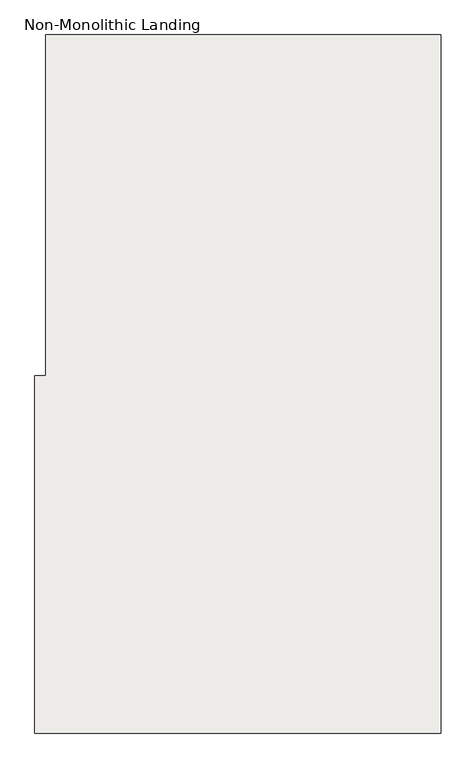
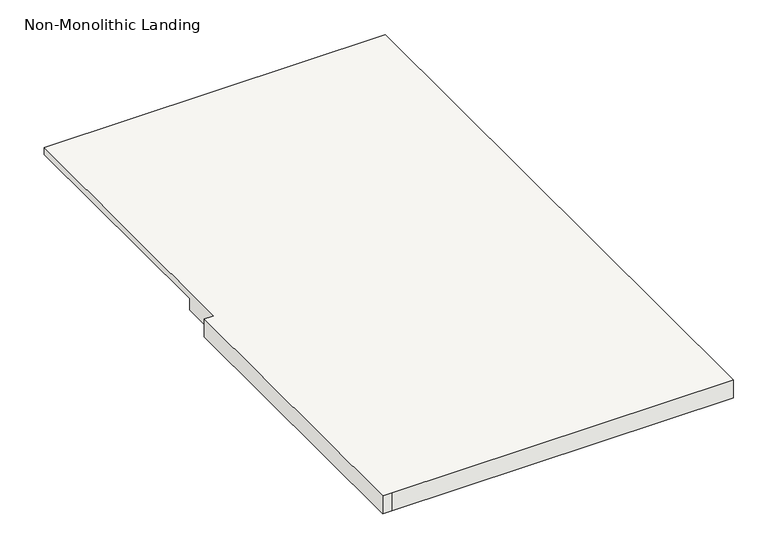
"""IFC4 building model written with IfcOpenShell, lengths in millimetres: slab geometry, Non-Monolithic Landing."""

from ifc_helpers import new_model, si_unit, origin, place, context, project, spatial, faceted_brep, source, transform, mapped, element, save


def non_monolithic_landing_dc928896(model_context):
    return source(origin(), model_context, "Body", "Brep", [
        faceted_brep([(-2950.6837185, -6386.6877785, 1581.15), (-2925.2837185, -6386.6877785, 1555.75), (-2925.2837185, -7060.9366292, 1555.75), (-2950.6837185, -7060.9366292, 1581.15), (-2950.6837185, -7174.0877785, 1600.2), (-2976.0837185, -7174.0877785, 1600.2), (-2976.0837185, -8000.7366292, 1600.2), (-2950.6837185, -8000.7366292, 1600.2), (-2036.2837185, -8000.7366292, 1600.2), (-2036.2837185, -6386.6877785, 1600.2), (-2950.6837185, -6386.6877785, 1600.2), (-2925.2837185, -7060.9366292, 1549.4), (-2925.2837185, -6386.6877785, 1549.4), (-2036.2837185, -6386.6877785, 1549.4), (-2036.2837185, -8000.7366292, 1549.4), (-2950.6837185, -8000.7366292, 1549.4), (-2976.0837185, -8000.7366292, 1549.4), (-2976.0837185, -7174.0877785, 1549.4), (-2950.6837185, -7174.0877785, 1549.4), (-2950.6837185, -7060.9366292, 1549.4)], [[[0, 1, 2, 3]], [[4, 5, 6, 7, 8, 9, 10]], [[11, 12, 13, 14, 15, 16, 17, 18, 19]], [[12, 11, 2, 1]], [[11, 19, 3, 2]], [[4, 10, 0, 3, 19, 18]], [[5, 4, 18, 17]], [[6, 5, 17, 16]], [[7, 6, 16, 15]], [[8, 7, 15, 14]], [[9, 8, 14, 13]], [[10, 9, 13, 12, 1, 0]]]),
    ])


if __name__ == "__main__":
    model = new_model("IFC4")
    model_context = context("Model", 3, world=origin())
    ifc_project = project(units=[si_unit("LENGTHUNIT", "METRE", prefix="MILLI")], contexts=[model_context])
    site = spatial("IfcSite", under=ifc_project)
    building = spatial("IfcBuilding", under=site)
    placement = place(None, origin())
    non_monolithic_landing_shape = non_monolithic_landing_dc928896(model_context)
    element("IfcSlab", 1, ObjectType="Non-Monolithic Landing", at=placement, inside=building, context=model_context, shape_type="MappedRepresentation", body=[
        mapped(non_monolithic_landing_shape, transform((0.0, 0.0, 0.0), x_axis=(1.0, 0.0, 0.0), y_axis=(0.0, 1.0, 0.0), z_axis=(0.0, 0.0, 1.0))),
    ])
    save(model, "model.ifc")
